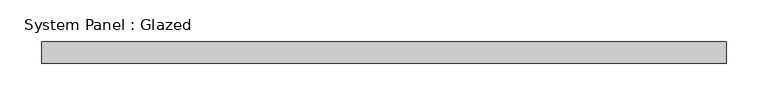
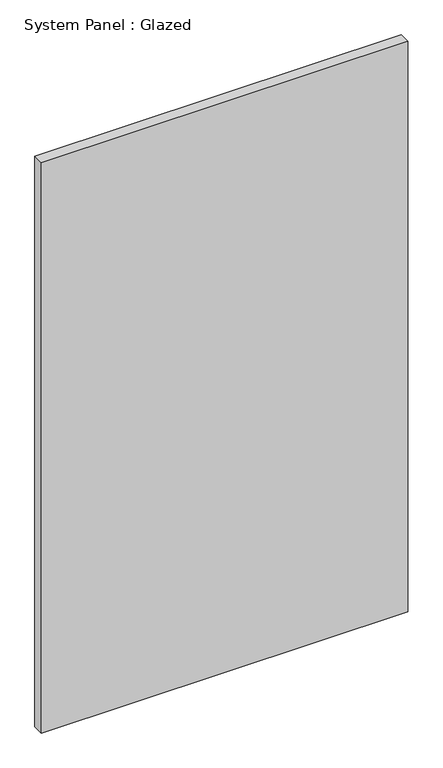
"""IFC4 building model written with IfcOpenShell, lengths in millimetres: plate geometry, System Panel : Glazed."""

from ifc_helpers import new_model, si_unit, origin, origin_with_axes, place, context, project, spatial, polyline, outline, extrude, source, transform, mapped, element, save


def system_panel_glazed_44ef0770(model_context):
    return source(origin(), model_context, "Body", "SweptSolid", [
        extrude(outline(polyline([(409.575, 19.05), (-409.575, 19.05), (-409.575, 44.45), (409.575, 44.45), (409.575, 19.05)])), origin_with_axes(), (0.0, 0.0, 1.0), 1348.7058851),
    ])


if __name__ == "__main__":
    model = new_model("IFC4")
    model_context = context("Model", 3, world=origin())
    ifc_project = project(units=[si_unit("LENGTHUNIT", "METRE", prefix="MILLI")], contexts=[model_context])
    site = spatial("IfcSite", under=ifc_project)
    building = spatial("IfcBuilding", under=site)
    placement = place(None, origin())
    system_panel_glazed_shape = system_panel_glazed_44ef0770(model_context)
    element("IfcPlate", 1, ObjectType="System Panel : Glazed", at=placement, inside=building, context=model_context, shape_type="MappedRepresentation", body=[
        mapped(system_panel_glazed_shape, transform((0.0, 0.0, 0.0), x_axis=(1.0, 0.0, 0.0), y_axis=(0.0, 1.0, 0.0), z_axis=(0.0, 0.0, 1.0))),
    ])
    save(model, "model.ifc")

# Revit data of these elements
# Type "System Panel : Glazed"
#   Construction Type Id = "GSP4R"
#   Analytic Construction = "1/8 in Pilkington single glazing"
#   Visual Light Transmittance = 0.9
#   Solar Heat Gain Coefficient = 0.86
#   Heat Transfer Coefficient (U) = 1.18115 BTU/(h·ft²·°F)
#   Define Thermal Properties by = 1
# Element 1 (IfcPlate, "System Panel : Glazed")
#   Materials on its faces: "Glass"
# Materials
#   "Glass": class "Glass", colour RGB 0 128 192, transparency 0.75, Description = "Soda Lime Glass", Cost = 0
